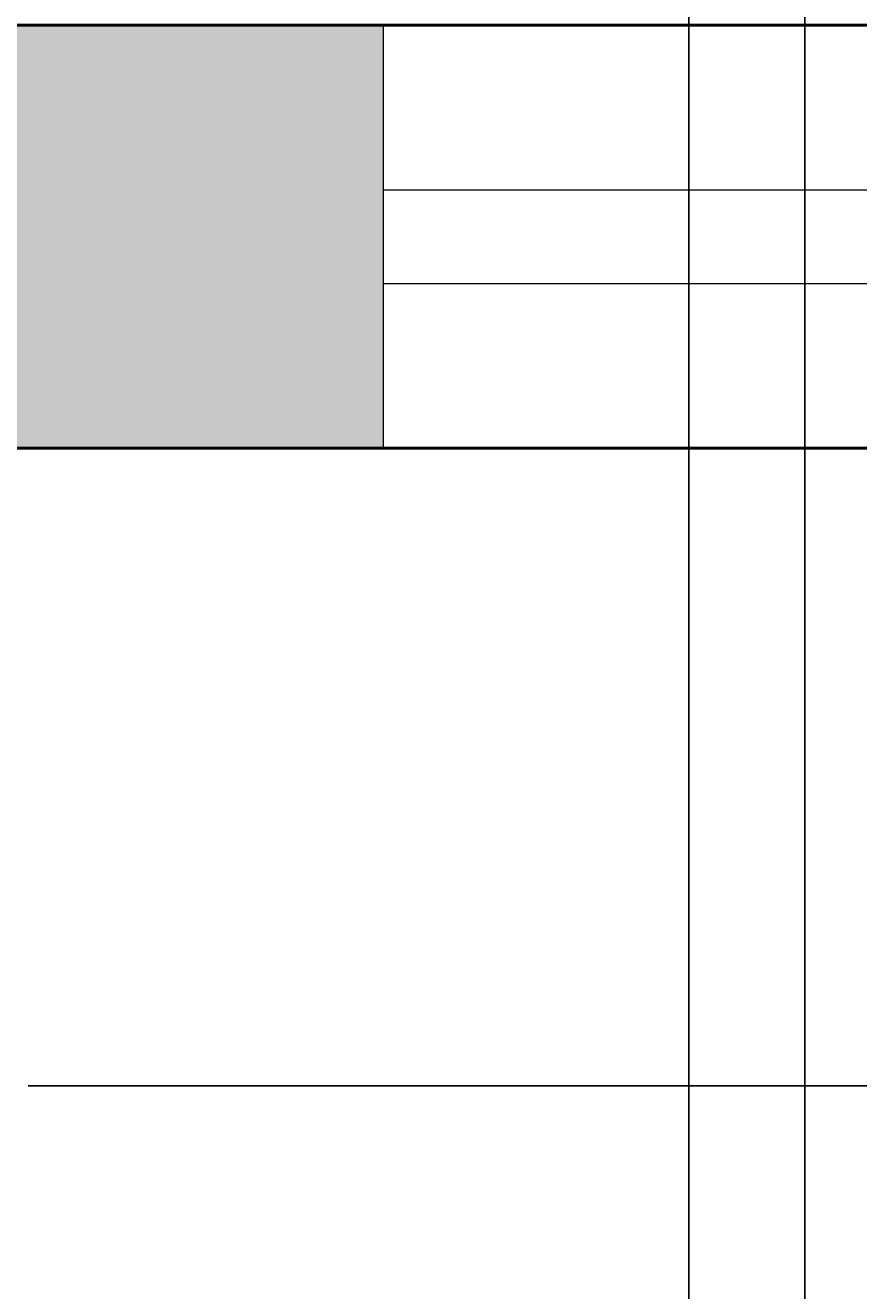
# Model space of a CAD drawing. Units: inches. Extents: x 2231 to 2461, y 2045 to 2455.
# Tile 76 of 95: x 2278 to 2296, y 2409 to 2436. Entities that reach past the tile are written whole.
import ezdxf

# ---------------------------------------------------------------- set-up
doc = ezdxf.new("R2010")
doc.units = ezdxf.units.IN
for name, color, linetype, lineweight in [('A-ANNO-DIMS', 2, 'Continuous', 18), ('A-GLAZ', 4, 'Continuous', 18), ('A-WALL', 7, 'Continuous', 50)]:
    doc.layers.add(name, color=color, linetype=linetype, lineweight=lineweight)
doc.layers.add('A-WALL-PATT', color=18, linetype='Continuous', lineweight=13, true_color=0x000000)
doc.styles.get("Standard").update_dxf_attribs({"font": 'arial.ttf'})
doc.dimstyles.get("Standard").update_dxf_attribs({"dimtxt": 0.18, "dimasz": 0.18, "dimexe": 0.18, "dimexo": 0.0625, "dimgap": 0.09, "dimtad": 0, "dimtih": 1, "dimtoh": 1, "dimdec": 4, "dimzin": 0, "dimdsep": 46, "dimtxsty": 'Standard', "dimcen": 0.09, "dimadec": 0, "dimazin": 0, "dimtfac": 1, "dimtdec": 4, "dimtofl": 0, "dimtmove": 0, "dimatfit": 3, "dimfxl": 1, "dimtolj": 1, "dimtzin": 0, "dimarcsym": 0})

# ---------------------------------------------------------------- blocks, each defined once
blk = doc.blocks.new('WIN-48IN')
for p, q in [((0, 0), (0, 9)), ((0, 5.5), (48, 5.5)), ((0, 3.5), (48, 3.5))]:
    blk.add_line(p, q)
blk = doc.blocks.new('*D35')
at = {"layer": 'A-ANNO-DIMS', "color": 0, "lineweight": -2, "transparency": 16777216}
for p, q in [((2258.794, 2426.895), (2258.794, 2454.645)), ((2368.794, 2426.895), (2368.794, 2454.645)), ((2258.974, 2454.465), (2313.513, 2454.465)), ((2368.614, 2454.465), (2314.074, 2454.465))]:
    blk.add_line(p, q, dxfattribs=at)
at = {"layer": 'A-ANNO-DIMS', "color": 0, "transparency": 16777216}
for points in [[(2258.974, 2454.495), (2258.974, 2454.435), (2258.794, 2454.465)], [(2368.614, 2454.495), (2368.614, 2454.435), (2368.794, 2454.465)]]:
    blk.add_solid(points, dxfattribs=at)
at = {"layer": 'Defpoints', "color": 0, "transparency": 16777216}
for p in [(2368.794, 2454.465), (2258.794, 2426.833), (2368.794, 2426.833)]:
    blk.add_point(p, dxfattribs=at)
at = {"layer": 'A-ANNO-DIMS', "color": 0, "transparency": 16777216, "insert": (2313.794, 2454.465), "char_height": 0.18, "attachment_point": 5}
blk.add_mtext('\\A1;110', dxfattribs=at)
blk = doc.blocks.new('*D47')
at = {"layer": 'A-ANNO-DIMS', "color": 0, "lineweight": -2, "transparency": 16777216}
for p, q in [((2258.794, 2182.895), (2258.794, 2454.645)), ((2294.794, 2182.895), (2294.794, 2454.645)), ((2258.974, 2454.465), (2276.575, 2454.465)), ((2294.614, 2454.465), (2277.012, 2454.465))]:
    blk.add_line(p, q, dxfattribs=at)
at = {"layer": 'A-ANNO-DIMS', "color": 0, "transparency": 16777216}
for points in [[(2258.974, 2454.495), (2258.974, 2454.435), (2258.794, 2454.465)], [(2294.614, 2454.495), (2294.614, 2454.435), (2294.794, 2454.465)]]:
    blk.add_solid(points, dxfattribs=at)
at = {"layer": 'Defpoints', "color": 0, "transparency": 16777216}
for p in [(2294.794, 2454.465), (2258.794, 2182.833), (2294.794, 2182.833)]:
    blk.add_point(p, dxfattribs=at)
at = {"layer": 'A-ANNO-DIMS', "color": 0, "transparency": 16777216, "insert": (2276.794, 2454.465), "char_height": 0.18, "attachment_point": 5}
blk.add_mtext('\\A1;36', dxfattribs=at)
blk = doc.blocks.new('*D62')
at = {"layer": 'A-ANNO-DIMS', "color": 0, "lineweight": -2, "transparency": 16777216}
for p, q in [((2262.321, 2255.176), (2262.321, 2454.645)), ((2292.321, 2253.176), (2292.321, 2454.645)), ((2262.501, 2454.465), (2277.102, 2454.465)), ((2292.141, 2454.465), (2277.539, 2454.465))]:
    blk.add_line(p, q, dxfattribs=at)
at = {"layer": 'A-ANNO-DIMS', "color": 0, "transparency": 16777216}
for points in [[(2262.501, 2454.495), (2262.501, 2454.435), (2262.321, 2454.465)], [(2292.141, 2454.495), (2292.141, 2454.435), (2292.321, 2454.465)]]:
    blk.add_solid(points, dxfattribs=at)
at = {"layer": 'Defpoints', "color": 0, "transparency": 16777216}
for p in [(2292.321, 2454.465), (2262.321, 2255.114), (2292.321, 2253.114)]:
    blk.add_point(p, dxfattribs=at)
at = {"layer": 'A-ANNO-DIMS', "color": 0, "transparency": 16777216, "insert": (2277.321, 2454.465), "char_height": 0.18, "attachment_point": 5}
blk.add_mtext('\\A1;30', dxfattribs=at)
blk = doc.blocks.new('*D68')
at = {"layer": 'A-ANNO-DIMS', "color": 0, "lineweight": -2, "transparency": 16777216}
for p, q in [((2285.882, 2426.833), (2460.606, 2426.833)), ((2460.426, 2426.653), (2460.426, 2420.225)), ((2460.426, 2413.433), (2460.426, 2419.861)), ((2278.251, 2413.253), (2460.606, 2413.253))]:
    blk.add_line(p, q, dxfattribs=at)
at = {"layer": 'A-ANNO-DIMS', "color": 0, "transparency": 16777216}
for points in [[(2460.396, 2426.653), (2460.456, 2426.653), (2460.426, 2426.833)], [(2460.396, 2413.433), (2460.456, 2413.433), (2460.426, 2413.253)]]:
    blk.add_solid(points, dxfattribs=at)
at = {"layer": 'Defpoints', "color": 0, "transparency": 16777216}
for p in [(2285.82, 2426.833), (2460.426, 2426.833), (2278.188, 2413.253)]:
    blk.add_point(p, dxfattribs=at)
at = {"layer": 'A-ANNO-DIMS', "color": 0, "transparency": 16777216, "insert": (2460.426, 2420.043), "char_height": 0.18, "attachment_point": 5}
blk.add_mtext('\\A1;13.58', dxfattribs=at)

msp = doc.modelspace()

# ---------------------------------------------------------------- hatches: boundary and pattern name
at = {"layer": 'A-WALL-PATT'}
h = msp.add_hatch(color=256, dxfattribs=at)
h.dxf.hatch_style = 1
h.paths.add_polyline_path([(2441.7935, 2269.1535), (2432.7935, 2269.1535), (2432.7935, 2186.8328), (2396.7935, 2186.8328), (2396.7935, 2286.8328), (2394.7935, 2286.8328), (2394.7935, 2186.8328), (2334.7935, 2186.8328), (2334.7935, 2182.8328), (2432.7935, 2182.8328), (2432.7935, 2072.8328), (2416.6639, 2072.8328), (2416.6639, 2063.8328), (2441.7935, 2063.8328)])
h.paths.add_polyline_path([(2368.6639, 2072.8328), (2367.04, 2072.8328), (2330.7942, 2072.8328), (2330.7397, 2063.8328), (2368.6639, 2063.8328)])
h.paths.add_polyline_path([(2300.7392, 2068.3328), (2300.7392, 2072.8328), (2298.7935, 2072.8328), (2294.7935, 2072.8328), (2258.7935, 2072.8328), (2258.7935, 2120.8328), (2294.7935, 2120.8328), (2298.7935, 2120.8328), (2298.7935, 2128.8328), (2294.7935, 2128.8328), (2294.7935, 2124.8328), (2258.7935, 2124.8328), (2258.7935, 2182.8328), (2294.7935, 2182.8328), (2294.7935, 2174.8328), (2298.7935, 2174.8328), (2298.7935, 2182.8328), (2304.7935, 2182.8328), (2304.7935, 2186.8328), (2258.7935, 2186.8328), (2258.7935, 2221.999), (2249.7935, 2221.999), (2249.7935, 2063.8328), (2300.7392, 2063.8328)])
h.paths.add_polyline_path([(2391.9338, 2435.8328), (2333.82, 2435.8328), (2333.82, 2426.8328), (2368.7935, 2426.8328), (2368.7935, 2374.9508), (2368.7935, 2370.8328), (2372.3935, 2370.8328), (2372.7935, 2370.8328), (2372.7935, 2426.8328), (2391.9338, 2426.8328)])
h.paths.add_polyline_path([(2441.7935, 2435.8328), (2415.9338, 2435.8328), (2415.9338, 2426.8328), (2432.7935, 2426.8328), (2432.7935, 2334.8328), (2372.7935, 2334.8328), (2372.7935, 2346.8328), (2368.7935, 2346.8328), (2368.7935, 2306.8328), (2360.7935, 2306.8328), (2360.7935, 2302.8328), (2368.7935, 2302.8328), (2372.7935, 2302.8328), (2372.7935, 2330.8328), (2432.7935, 2330.8328), (2432.7935, 2317.1535), (2441.7935, 2317.1535)])
h.paths.add_polyline_path([(2285.82, 2435.8328), (2249.7935, 2435.8328), (2249.7935, 2269.999), (2258.7935, 2269.999), (2258.7935, 2302.8328), (2318.8168, 2302.8328), (2330.7935, 2302.8328), (2330.7935, 2306.8328), (2258.7935, 2306.8328), (2258.7935, 2426.8328), (2285.82, 2426.8328)])

# ---------------------------------------------------------------- linework, layer by layer
at = {"layer": 'A-WALL'}
msp.add_line((2258.7935, 2426.8328), (2368.7935, 2426.8328), dxfattribs=at)
msp.add_lwpolyline([(2300.7392, 2063.8328), (2249.7935, 2063.8328), (2249.7935, 2435.8328), (2441.7935, 2435.8328), (2441.7935, 2063.8328), (2330.7397, 2063.8328)], dxfattribs=at)

# ---------------------------------------------------------------- block references
at = {"layer": 'A-GLAZ'}
msp.add_blockref('WIN-48IN', (2285.82, 2426.833), dxfattribs=at)

# ---------------------------------------------------------------- dimensions: what is measured, and where the dimension line sits
at = {"layer": 'A-ANNO-DIMS'}
for base, p1, p2, picture, middle in [((2368.7935, 2454.4653), (2258.7935, 2426.8328), (2368.7935, 2426.8328), '*D35', (2313.7935, 2454.4653)), ((2294.7935, 2454.4653), (2258.7935, 2182.8328), (2294.7935, 2182.8328), '*D47', (2276.7935, 2454.4653)), ((2292.3207, 2454.4653), (2262.3207, 2255.1137), (2292.3207, 2253.1137), '*D62', (2277.3207, 2454.4653))]:
    dim = msp.add_linear_dim(base=base, p1=p1, p2=p2, dimstyle='Standard', override={"dimdec": 0, "dimlfac": 1, "dimrnd": 0, "dimzin": 0, "dimdsep": 46, "dimlunit": 2}, dxfattribs=at)
    dim.commit()
    dim.dimension.update_dxf_attribs({"geometry": picture, "text_midpoint": middle})
dim = msp.add_linear_dim(base=(2460.426, 2426.8328), p1=(2278.1881, 2413.2534), p2=(2285.82, 2426.8328), angle=90, dimstyle='Standard', override={"dimdec": 2, "dimlfac": 1, "dimrnd": 0, "dimzin": 0, "dimdsep": 46, "dimlunit": 2}, dxfattribs=at)
dim.commit()
dim.dimension.update_dxf_attribs({"geometry": '*D68', "text_midpoint": (2460.426, 2420.0431)})

doc.saveas('drawing.dxf')
